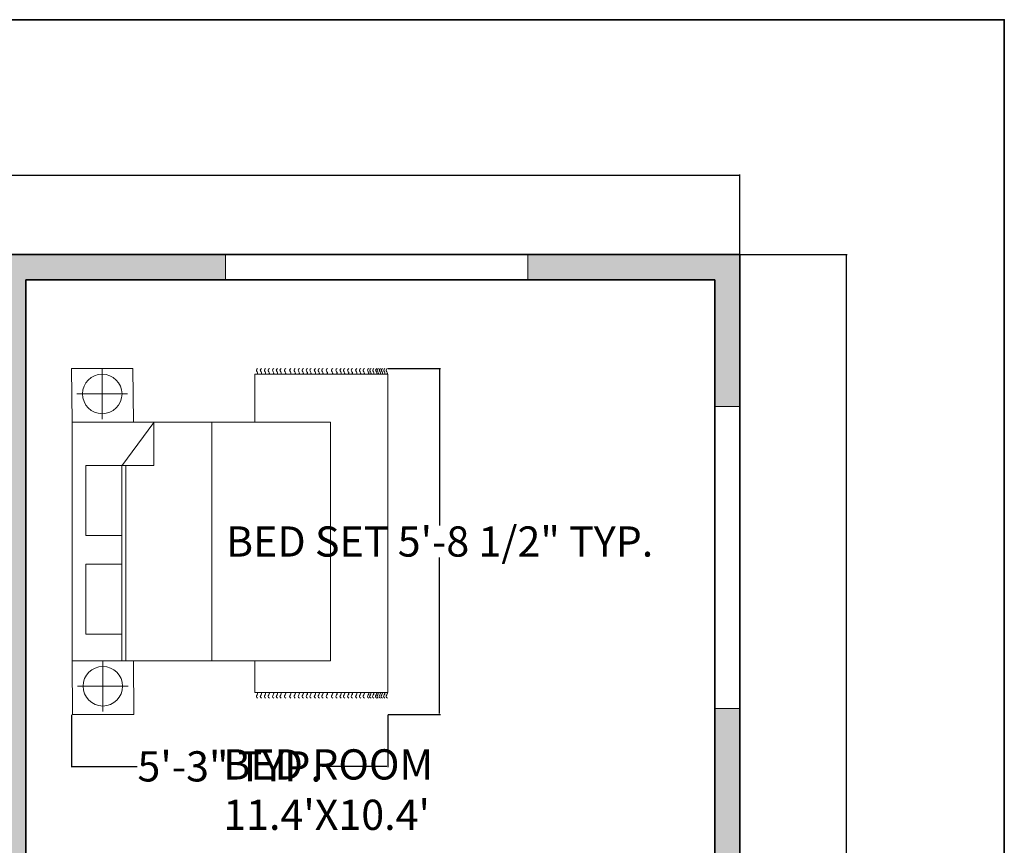
# Model space of a CAD drawing. Units: inches. Extents: x 717 to 1167, y 2046 to 2594.
# Tile 6 of 6: x 972 to 1167, y 2430 to 2594. Entities that reach past the tile are written whole.
import ezdxf

# ---------------------------------------------------------------- set-up
doc = ezdxf.new("R2010")
doc.units = ezdxf.units.IN
doc.header["$MEASUREMENT"] = 0
for name, color, linetype, lineweight in [('A-ANNO-DIMS', 2, 'Continuous', 18), ('A-ANNO-TTLB', 7, 'Continuous', 35), ('A-AREA-IDEN', 7, 'Continuous', 18), ('A-FURN', 8, 'Continuous', 18), ('A-GLAZ', 4, 'Continuous', 18), ('A-WALL', 7, 'Continuous', 35), ('A-WALL-PATT', 140, 'Continuous', 13)]:
    doc.layers.add(name, color=color, linetype=linetype, lineweight=lineweight)
doc.styles.get("Standard").update_dxf_attribs({"font": 'arial.ttf'})
doc.dimstyles.get("Standard").update_dxf_attribs({"dimtxt": 6, "dimasz": 0.18, "dimexe": 0.18, "dimexo": 0.0625, "dimgap": 0.09, "dimtad": 0, "dimtih": 1, "dimtoh": 1, "dimdec": 1, "dimzin": 0, "dimdsep": 46, "dimlunit": 3, "dimtxsty": 'Standard', "dimcen": 0.09, "dimadec": 0, "dimazin": 0, "dimtfac": 1, "dimtdec": 1, "dimtofl": 0, "dimtmove": 0, "dimatfit": 3, "dimfxl": 1, "dimtolj": 1, "dimtzin": 0, "dimarcsym": 0})

# ---------------------------------------------------------------- blocks, each defined once
blk = doc.blocks.new('*D4')
at = {"layer": 'A-ANNO-DIMS', "color": 0, "lineweight": -2, "transparency": 16777216}
for p, q in [((754.71, 2547.63), (754.71, 2563.46)), ((754.89, 2563.28), (929.54, 2563.28)), ((1114.53, 2563.28), (939.89, 2563.28)), ((1114.71, 2547.63), (1114.71, 2563.46))]:
    blk.add_line(p, q, dxfattribs=at)
at = {"layer": 'A-ANNO-DIMS', "color": 0, "transparency": 16777216}
for points in [[(754.89, 2563.31), (754.89, 2563.25), (754.71, 2563.28)], [(1114.53, 2563.31), (1114.53, 2563.25), (1114.71, 2563.28)]]:
    blk.add_solid(points, dxfattribs=at)
at = {"layer": 'Defpoints', "color": 0, "transparency": 16777216}
for p in [(1114.71, 2563.28), (754.71, 2547.57), (1114.71, 2547.57)]:
    blk.add_point(p, dxfattribs=at)
at = {"layer": 'A-ANNO-DIMS', "color": 0, "transparency": 16777216, "insert": (934.71, 2563.28), "char_height": 6, "attachment_point": 5}
blk.add_mtext("\\A1;30'", dxfattribs=at)
blk = doc.blocks.new('*D5')
at = {"layer": 'A-ANNO-DIMS', "color": 0, "lineweight": -2, "transparency": 16777216}
for p, q in [((1114.78, 2547.57), (1135.98, 2547.57)), ((1135.8, 2547.39), (1135.8, 2316.73)), ((1135.8, 2079.75), (1135.8, 2310.41)), ((1114.78, 2079.57), (1135.98, 2079.57))]:
    blk.add_line(p, q, dxfattribs=at)
at = {"layer": 'A-ANNO-DIMS', "color": 0, "transparency": 16777216}
for points in [[(1135.77, 2547.39), (1135.83, 2547.39), (1135.8, 2547.57)], [(1135.77, 2079.75), (1135.83, 2079.75), (1135.8, 2079.57)]]:
    blk.add_solid(points, dxfattribs=at)
at = {"layer": 'Defpoints', "color": 0, "transparency": 16777216}
for p in [(1114.71, 2547.57), (1114.71, 2079.57), (1135.8, 2079.57)]:
    blk.add_point(p, dxfattribs=at)
at = {"layer": 'A-ANNO-DIMS', "color": 0, "transparency": 16777216, "insert": (1135.8, 2313.57), "char_height": 6, "attachment_point": 5}
blk.add_mtext("\\A1;39'", dxfattribs=at)
blk = doc.blocks.new('BED-DOUBLE-WITH-NIGHTSTANDS')
for p, q in [((6.09, 68.68), (6.09, 58.62)), ((36.42, 67.59), (62.78, 67.59)), ((36.42, 58.05), (36.42, 67.59)), ((62.78, 67.59), (62.78, 4.35)), ((1.07, 63.65), (11.12, 63.65)), ((9.97, 49.39), (16.32, 58)), ((16.32, 49.44), (16.32, 58)), ((27.82, 58.05), (27.82, 10.63)), ((9.97, 49.44), (16.32, 49.44)), ((9.97, 49.39), (9.97, 10.63)), ((10.78, 49.44), (10.78, 10.63)), ((6.2, 10.63), (6.2, 0.57)), ((36.42, 4.35), (36.42, 10.65)), ((1.17, 5.6), (11.22, 5.6)), ((62.78, 4.35), (36.42, 4.35))]:
    blk.add_line(p, q)
for points in [[(12.29, 58.05), (12.19, 68.68), (0, 68.68), (0.1, 58.05)], [(0.1, 58.05), (51.42, 58.05), (51.42, 10.63), (0.1, 10.63)], [(2.8, 49.44), (9.97, 49.44), (9.97, 35.55), (2.8, 35.55)], [(2.8, 29.88), (9.97, 29.88), (9.97, 15.98), (2.8, 15.98)], [(12.39, 0), (12.29, 10.63), (0.1, 10.63), (0.21, 0)]]:
    blk.add_lwpolyline(points, close=True)
for centre in [(6.09, 63.65), (6.2, 5.6)]:
    blk.add_circle(centre, 3.92)
for points, knots in [([(36.95, 68.71), (36.83, 68.61), (36.59, 68.42), (36.83, 68.08), (37, 67.8), (36.89, 67.65), (36.85, 67.58)], [0, 0, 0, 0, 0.400747, 0.791423, 1.067667, 1.29709, 1.29709, 1.29709, 1.29709]), ([(37.73, 68.71), (37.61, 68.61), (37.37, 68.42), (37.61, 68.08), (37.78, 67.8), (37.67, 67.65), (37.62, 67.58)], [0, 0, 0, 0, 0.400747, 0.791423, 1.067667, 1.29709, 1.29709, 1.29709, 1.29709]), ([(38.54, 68.71), (38.42, 68.61), (38.18, 68.42), (38.42, 68.08), (38.59, 67.8), (38.49, 67.65), (38.44, 67.58)], [0, 0, 0, 0, 0.400747, 0.791423, 1.067667, 1.29709, 1.29709, 1.29709, 1.29709]), ([(39.27, 68.71), (39.15, 68.61), (38.91, 68.42), (39.15, 68.08), (39.32, 67.8), (39.22, 67.65), (39.17, 67.58)], [0, 0, 0, 0, 0.400747, 0.791423, 1.067667, 1.29709, 1.29709, 1.29709, 1.29709]), ([(40.15, 68.71), (40.03, 68.61), (39.79, 68.42), (40.03, 68.08), (40.2, 67.8), (40.1, 67.65), (40.05, 67.58)], [0, 0, 0, 0, 0.400747, 0.791423, 1.067667, 1.29709, 1.29709, 1.29709, 1.29709]), ([(40.91, 68.71), (40.78, 68.61), (40.54, 68.42), (40.78, 68.08), (40.96, 67.8), (40.85, 67.65), (40.8, 67.58)], [0, 0, 0, 0, 0.400747, 0.791423, 1.067667, 1.29709, 1.29709, 1.29709, 1.29709]), ([(41.63, 68.71), (41.51, 68.61), (41.27, 68.42), (41.51, 68.08), (41.69, 67.8), (41.58, 67.65), (41.53, 67.58)], [0, 0, 0, 0, 0.400747, 0.791423, 1.067667, 1.29709, 1.29709, 1.29709, 1.29709]), ([(42.52, 68.71), (42.39, 68.61), (42.16, 68.42), (42.39, 68.08), (42.57, 67.8), (42.46, 67.65), (42.41, 67.58)], [0, 0, 0, 0, 0.400747, 0.791423, 1.067667, 1.29709, 1.29709, 1.29709, 1.29709]), ([(43.55, 68.71), (43.43, 68.61), (43.19, 68.42), (43.43, 68.08), (43.6, 67.8), (43.5, 67.65), (43.45, 67.58)], [0, 0, 0, 0, 0.400747, 0.791423, 1.067667, 1.29709, 1.29709, 1.29709, 1.29709]), ([(44.43, 68.71), (44.31, 68.61), (44.07, 68.42), (44.31, 68.08), (44.49, 67.8), (44.38, 67.65), (44.33, 67.58)], [0, 0, 0, 0, 0.400747, 0.791423, 1.067667, 1.29709, 1.29709, 1.29709, 1.29709]), ([(45.25, 68.71), (45.13, 68.61), (44.89, 68.42), (45.13, 68.08), (45.3, 67.8), (45.2, 67.65), (45.15, 67.58)], [0, 0, 0, 0, 0.400747, 0.791423, 1.067667, 1.29709, 1.29709, 1.29709, 1.29709]), ([(46.03, 68.71), (45.91, 68.61), (45.67, 68.42), (45.91, 68.08), (46.08, 67.8), (45.97, 67.65), (45.92, 67.58)], [0, 0, 0, 0, 0.400747, 0.791423, 1.067667, 1.29709, 1.29709, 1.29709, 1.29709]), ([(46.84, 68.71), (46.72, 68.61), (46.48, 68.42), (46.72, 68.08), (46.9, 67.8), (46.79, 67.65), (46.74, 67.58)], [0, 0, 0, 0, 0.400747, 0.791423, 1.067667, 1.29709, 1.29709, 1.29709, 1.29709]), ([(47.57, 68.71), (47.45, 68.61), (47.21, 68.42), (47.45, 68.08), (47.62, 67.8), (47.52, 67.65), (47.47, 67.58)], [0, 0, 0, 0, 0.400747, 0.791423, 1.067667, 1.29709, 1.29709, 1.29709, 1.29709]), ([(48.45, 68.71), (48.33, 68.61), (48.09, 68.42), (48.33, 68.08), (48.51, 67.8), (48.4, 67.65), (48.35, 67.58)], [0, 0, 0, 0, 0.400747, 0.791423, 1.067667, 1.29709, 1.29709, 1.29709, 1.29709]), ([(49.21, 68.71), (49.08, 68.61), (48.85, 68.42), (49.08, 68.08), (49.26, 67.8), (49.15, 67.65), (49.1, 67.58)], [0, 0, 0, 0, 0.400747, 0.791423, 1.067667, 1.29709, 1.29709, 1.29709, 1.29709]), ([(49.93, 68.71), (49.81, 68.61), (49.57, 68.42), (49.81, 68.08), (49.99, 67.8), (49.88, 67.65), (49.83, 67.58)], [0, 0, 0, 0, 0.400747, 0.791423, 1.067667, 1.29709, 1.29709, 1.29709, 1.29709]), ([(50.82, 68.71), (50.69, 68.61), (50.46, 68.42), (50.69, 68.08), (50.87, 67.8), (50.76, 67.65), (50.71, 67.58)], [0, 0, 0, 0, 0.400747, 0.791423, 1.067667, 1.29709, 1.29709, 1.29709, 1.29709]), ([(51.85, 68.71), (51.73, 68.61), (51.49, 68.42), (51.73, 68.08), (51.9, 67.8), (51.8, 67.65), (51.75, 67.58)], [0, 0, 0, 0, 0.400747, 0.791423, 1.067667, 1.29709, 1.29709, 1.29709, 1.29709]), ([(52.74, 68.71), (52.61, 68.61), (52.37, 68.42), (52.61, 68.08), (52.79, 67.8), (52.68, 67.65), (52.63, 67.58)], [0, 0, 0, 0, 0.400747, 0.791423, 1.067667, 1.29709, 1.29709, 1.29709, 1.29709]), ([(53.55, 68.71), (53.43, 68.61), (53.19, 68.42), (53.43, 68.08), (53.6, 67.8), (53.5, 67.65), (53.45, 67.58)], [0, 0, 0, 0, 0.400747, 0.791423, 1.067667, 1.29709, 1.29709, 1.29709, 1.29709]), ([(54.24, 68.71), (54.12, 68.61), (53.88, 68.42), (54.12, 68.08), (54.29, 67.8), (54.19, 67.65), (54.14, 67.58)], [0, 0, 0, 0, 0.400747, 0.791423, 1.067667, 1.29709, 1.29709, 1.29709, 1.29709]), ([(55.06, 68.71), (54.94, 68.61), (54.7, 68.42), (54.94, 68.08), (55.11, 67.8), (55, 67.65), (54.95, 67.58)], [0, 0, 0, 0, 0.400747, 0.791423, 1.067667, 1.29709, 1.29709, 1.29709, 1.29709]), ([(55.78, 68.71), (55.66, 68.61), (55.42, 68.42), (55.66, 68.08), (55.84, 67.8), (55.73, 67.65), (55.68, 67.58)], [0, 0, 0, 0, 0.400747, 0.791423, 1.067667, 1.29709, 1.29709, 1.29709, 1.29709]), ([(56.67, 68.71), (56.55, 68.61), (56.31, 68.42), (56.55, 68.08), (56.72, 67.8), (56.61, 67.65), (56.56, 67.58)], [0, 0, 0, 0, 0.400747, 0.791423, 1.067667, 1.29709, 1.29709, 1.29709, 1.29709]), ([(57.42, 68.71), (57.3, 68.61), (57.06, 68.42), (57.3, 68.08), (57.47, 67.8), (57.36, 67.65), (57.32, 67.58)], [0, 0, 0, 0, 0.400747, 0.791423, 1.067667, 1.29709, 1.29709, 1.29709, 1.29709]), ([(58.15, 68.71), (58.03, 68.61), (57.79, 68.42), (58.03, 68.08), (58.2, 67.8), (58.1, 67.66), (58.05, 67.59)], [0, 0, 0, 0, 0.400747, 0.791423, 1.067667, 1.283686, 1.283686, 1.283686, 1.283686]), ([(59.03, 68.71), (58.91, 68.61), (58.67, 68.42), (58.91, 68.08), (59.08, 67.8), (58.98, 67.66), (58.93, 67.59)], [0, 0, 0, 0, 0.400747, 0.791423, 1.067667, 1.283686, 1.283686, 1.283686, 1.283686]), ([(59.46, 68.71), (59.34, 68.61), (59.09, 68.42), (59.34, 68.08), (59.51, 67.8), (59.41, 67.66), (59.36, 67.59)], [0, 0, 0, 0, 0.402903, 0.794912, 1.071156, 1.287177, 1.287177, 1.287177, 1.287177]), ([(60.05, 68.71), (59.93, 68.61), (59.69, 68.42), (59.93, 68.08), (60.1, 67.8), (60, 67.66), (59.96, 67.59)], [0, 0, 0, 0, 0.400747, 0.791423, 1.067667, 1.283686, 1.283686, 1.283686, 1.283686]), ([(60.63, 68.71), (60.51, 68.61), (60.27, 68.42), (60.51, 68.08), (60.68, 67.8), (60.58, 67.66), (60.53, 67.59)], [0, 0, 0, 0, 0.400747, 0.791423, 1.067667, 1.283686, 1.283686, 1.283686, 1.283686]), ([(60.94, 68.71), (60.82, 68.61), (60.58, 68.42), (60.81, 68.08), (60.99, 67.8), (60.89, 67.66), (60.84, 67.59)], [0, 0, 0, 0, 0.400747, 0.791423, 1.067667, 1.283686, 1.283686, 1.283686, 1.283686]), ([(61.36, 68.71), (61.23, 68.61), (60.99, 68.42), (61.23, 68.08), (61.41, 67.8), (61.3, 67.65), (61.25, 67.58)], [0, 0, 0, 0, 0.400747, 0.791423, 1.067667, 1.29709, 1.29709, 1.29709, 1.29709]), ([(61.75, 68.71), (61.63, 68.61), (61.39, 68.42), (61.63, 68.08), (61.8, 67.8), (61.7, 67.65), (61.65, 67.58)], [0, 0, 0, 0, 0.400747, 0.791423, 1.067667, 1.29709, 1.29709, 1.29709, 1.29709]), ([(62.24, 68.71), (62.12, 68.61), (61.88, 68.42), (62.12, 68.08), (62.29, 67.8), (62.18, 67.65), (62.13, 67.58)], [0, 0, 0, 0, 0.400747, 0.791423, 1.067667, 1.29709, 1.29709, 1.29709, 1.29709]), ([(62.71, 68.71), (62.59, 68.61), (62.35, 68.42), (62.59, 68.08), (62.76, 67.8), (62.66, 67.65), (62.61, 67.58)], [0, 0, 0, 0, 0.400747, 0.791423, 1.067667, 1.29709, 1.29709, 1.29709, 1.29709]), ([(36.95, 3.23), (36.83, 3.32), (36.59, 3.52), (36.83, 3.86), (37, 4.14), (36.89, 4.29), (36.85, 4.35)], [0, 0, 0, 0, 0.400747, 0.791423, 1.067667, 1.29709, 1.29709, 1.29709, 1.29709]), ([(37.73, 3.23), (37.61, 3.32), (37.37, 3.52), (37.61, 3.86), (37.78, 4.14), (37.67, 4.29), (37.62, 4.35)], [0, 0, 0, 0, 0.400747, 0.791423, 1.067667, 1.29709, 1.29709, 1.29709, 1.29709]), ([(38.54, 3.23), (38.42, 3.32), (38.18, 3.52), (38.42, 3.86), (38.59, 4.14), (38.49, 4.29), (38.44, 4.35)], [0, 0, 0, 0, 0.400747, 0.791423, 1.067667, 1.29709, 1.29709, 1.29709, 1.29709]), ([(39.27, 3.23), (39.15, 3.32), (38.91, 3.52), (39.15, 3.86), (39.32, 4.14), (39.22, 4.29), (39.17, 4.35)], [0, 0, 0, 0, 0.400747, 0.791423, 1.067667, 1.29709, 1.29709, 1.29709, 1.29709]), ([(40.15, 3.23), (40.03, 3.32), (39.79, 3.52), (40.03, 3.86), (40.2, 4.14), (40.1, 4.29), (40.05, 4.35)], [0, 0, 0, 0, 0.400747, 0.791423, 1.067667, 1.29709, 1.29709, 1.29709, 1.29709]), ([(40.91, 3.23), (40.78, 3.32), (40.54, 3.52), (40.78, 3.86), (40.96, 4.14), (40.85, 4.29), (40.8, 4.35)], [0, 0, 0, 0, 0.400747, 0.791423, 1.067667, 1.29709, 1.29709, 1.29709, 1.29709]), ([(41.63, 3.23), (41.51, 3.32), (41.27, 3.52), (41.51, 3.86), (41.69, 4.14), (41.58, 4.29), (41.53, 4.35)], [0, 0, 0, 0, 0.400747, 0.791423, 1.067667, 1.29709, 1.29709, 1.29709, 1.29709]), ([(42.52, 3.23), (42.39, 3.32), (42.16, 3.52), (42.39, 3.86), (42.57, 4.14), (42.46, 4.29), (42.41, 4.35)], [0, 0, 0, 0, 0.400747, 0.791423, 1.067667, 1.29709, 1.29709, 1.29709, 1.29709]), ([(43.55, 3.23), (43.43, 3.32), (43.19, 3.52), (43.43, 3.86), (43.6, 4.14), (43.5, 4.29), (43.45, 4.35)], [0, 0, 0, 0, 0.400747, 0.791423, 1.067667, 1.29709, 1.29709, 1.29709, 1.29709]), ([(44.43, 3.23), (44.31, 3.32), (44.07, 3.52), (44.31, 3.86), (44.49, 4.14), (44.38, 4.29), (44.33, 4.35)], [0, 0, 0, 0, 0.400747, 0.791423, 1.067667, 1.29709, 1.29709, 1.29709, 1.29709]), ([(45.25, 3.23), (45.13, 3.32), (44.89, 3.52), (45.13, 3.86), (45.3, 4.14), (45.2, 4.29), (45.15, 4.35)], [0, 0, 0, 0, 0.400747, 0.791423, 1.067667, 1.29709, 1.29709, 1.29709, 1.29709]), ([(46.03, 3.23), (45.91, 3.32), (45.67, 3.52), (45.91, 3.86), (46.08, 4.14), (45.97, 4.29), (45.92, 4.35)], [0, 0, 0, 0, 0.400747, 0.791423, 1.067667, 1.29709, 1.29709, 1.29709, 1.29709]), ([(46.84, 3.23), (46.72, 3.32), (46.48, 3.52), (46.72, 3.86), (46.9, 4.14), (46.79, 4.29), (46.74, 4.35)], [0, 0, 0, 0, 0.400747, 0.791423, 1.067667, 1.29709, 1.29709, 1.29709, 1.29709]), ([(47.57, 3.23), (47.45, 3.32), (47.21, 3.52), (47.45, 3.86), (47.62, 4.14), (47.52, 4.29), (47.47, 4.35)], [0, 0, 0, 0, 0.400747, 0.791423, 1.067667, 1.29709, 1.29709, 1.29709, 1.29709]), ([(48.45, 3.23), (48.33, 3.32), (48.09, 3.52), (48.33, 3.86), (48.51, 4.14), (48.4, 4.29), (48.35, 4.35)], [0, 0, 0, 0, 0.400747, 0.791423, 1.067667, 1.29709, 1.29709, 1.29709, 1.29709]), ([(49.21, 3.23), (49.08, 3.32), (48.85, 3.52), (49.08, 3.86), (49.26, 4.14), (49.15, 4.29), (49.1, 4.35)], [0, 0, 0, 0, 0.400747, 0.791423, 1.067667, 1.29709, 1.29709, 1.29709, 1.29709]), ([(49.93, 3.23), (49.81, 3.32), (49.57, 3.52), (49.81, 3.86), (49.99, 4.14), (49.88, 4.29), (49.83, 4.35)], [0, 0, 0, 0, 0.400747, 0.791423, 1.067667, 1.29709, 1.29709, 1.29709, 1.29709]), ([(50.82, 3.23), (50.69, 3.32), (50.46, 3.52), (50.69, 3.86), (50.87, 4.14), (50.76, 4.29), (50.71, 4.35)], [0, 0, 0, 0, 0.400747, 0.791423, 1.067667, 1.29709, 1.29709, 1.29709, 1.29709]), ([(51.85, 3.23), (51.73, 3.32), (51.49, 3.52), (51.73, 3.86), (51.9, 4.14), (51.8, 4.29), (51.75, 4.35)], [0, 0, 0, 0, 0.400747, 0.791423, 1.067667, 1.29709, 1.29709, 1.29709, 1.29709]), ([(52.74, 3.23), (52.61, 3.32), (52.37, 3.52), (52.61, 3.86), (52.79, 4.14), (52.68, 4.29), (52.63, 4.35)], [0, 0, 0, 0, 0.400747, 0.791423, 1.067667, 1.29709, 1.29709, 1.29709, 1.29709]), ([(53.55, 3.23), (53.43, 3.32), (53.19, 3.52), (53.43, 3.86), (53.6, 4.14), (53.5, 4.29), (53.45, 4.35)], [0, 0, 0, 0, 0.400747, 0.791423, 1.067667, 1.29709, 1.29709, 1.29709, 1.29709]), ([(54.24, 3.23), (54.12, 3.32), (53.88, 3.52), (54.12, 3.86), (54.29, 4.14), (54.19, 4.29), (54.14, 4.35)], [0, 0, 0, 0, 0.400747, 0.791423, 1.067667, 1.29709, 1.29709, 1.29709, 1.29709]), ([(55.06, 3.23), (54.94, 3.32), (54.7, 3.52), (54.94, 3.86), (55.11, 4.14), (55, 4.29), (54.95, 4.35)], [0, 0, 0, 0, 0.400747, 0.791423, 1.067667, 1.29709, 1.29709, 1.29709, 1.29709]), ([(55.78, 3.23), (55.66, 3.32), (55.42, 3.52), (55.66, 3.86), (55.84, 4.14), (55.73, 4.29), (55.68, 4.35)], [0, 0, 0, 0, 0.400747, 0.791423, 1.067667, 1.29709, 1.29709, 1.29709, 1.29709]), ([(56.67, 3.23), (56.55, 3.32), (56.31, 3.52), (56.55, 3.86), (56.72, 4.14), (56.61, 4.29), (56.56, 4.35)], [0, 0, 0, 0, 0.400747, 0.791423, 1.067667, 1.29709, 1.29709, 1.29709, 1.29709]), ([(57.42, 3.23), (57.3, 3.32), (57.06, 3.52), (57.3, 3.86), (57.47, 4.14), (57.36, 4.29), (57.32, 4.35)], [0, 0, 0, 0, 0.400747, 0.791423, 1.067667, 1.29709, 1.29709, 1.29709, 1.29709]), ([(58.15, 3.23), (58.03, 3.32), (57.79, 3.52), (58.03, 3.86), (58.2, 4.14), (58.09, 4.29), (58.04, 4.35)], [0, 0, 0, 0, 0.400747, 0.791423, 1.067667, 1.29709, 1.29709, 1.29709, 1.29709]), ([(59.03, 3.23), (58.91, 3.32), (58.67, 3.52), (58.91, 3.86), (59.08, 4.14), (58.98, 4.29), (58.93, 4.35)], [0, 0, 0, 0, 0.400747, 0.791423, 1.067667, 1.29709, 1.29709, 1.29709, 1.29709]), ([(59.46, 3.23), (59.33, 3.32), (59.08, 3.51), (59.34, 3.86), (59.51, 4.14), (59.4, 4.29), (59.36, 4.35)], [0, 0, 0, 0, 0.407265, 0.802015, 1.07826, 1.307683, 1.307683, 1.307683, 1.307683]), ([(60.03, 3.23), (59.9, 3.32), (59.67, 3.52), (59.9, 3.86), (60.08, 4.14), (59.97, 4.29), (59.92, 4.35)], [0, 0, 0, 0, 0.400747, 0.791423, 1.067667, 1.29709, 1.29709, 1.29709, 1.29709]), ([(60.6, 3.23), (60.48, 3.32), (60.24, 3.52), (60.48, 3.86), (60.65, 4.14), (60.54, 4.29), (60.5, 4.35)], [0, 0, 0, 0, 0.400747, 0.791423, 1.067667, 1.29709, 1.29709, 1.29709, 1.29709]), ([(60.91, 3.23), (60.79, 3.32), (60.55, 3.52), (60.79, 3.86), (60.96, 4.14), (60.85, 4.29), (60.81, 4.35)], [0, 0, 0, 0, 0.400747, 0.791423, 1.067667, 1.29709, 1.29709, 1.29709, 1.29709]), ([(61.33, 3.23), (61.21, 3.32), (60.97, 3.52), (61.21, 3.86), (61.38, 4.14), (61.27, 4.29), (61.22, 4.35)], [0, 0, 0, 0, 0.400747, 0.791423, 1.067667, 1.29709, 1.29709, 1.29709, 1.29709]), ([(61.72, 3.23), (61.6, 3.32), (61.36, 3.52), (61.6, 3.86), (61.78, 4.14), (61.67, 4.29), (61.62, 4.35)], [0, 0, 0, 0, 0.400747, 0.791423, 1.067667, 1.29709, 1.29709, 1.29709, 1.29709]), ([(62.21, 3.23), (62.09, 3.32), (61.85, 3.52), (62.09, 3.86), (62.26, 4.14), (62.15, 4.29), (62.11, 4.35)], [0, 0, 0, 0, 0.400747, 0.791423, 1.067667, 1.29709, 1.29709, 1.29709, 1.29709]), ([(62.71, 3.23), (62.59, 3.32), (62.35, 3.52), (62.59, 3.86), (62.76, 4.14), (62.66, 4.29), (62.61, 4.35)], [0, 0, 0, 0, 0.400747, 0.791423, 1.067667, 1.29709, 1.29709, 1.29709, 1.29709])]:
    blk.add_open_spline(points, degree=3, knots=knots)
blk = doc.blocks.new('WINDOW-60IN')
for p, q in [((0, 5), (0, 0)), ((60, 5), (0, 5)), ((60, 0), (60, 5)), ((0, 0), (60, 0))]:
    blk.add_line(p, q)
blk = doc.blocks.new('*D17')
at = {"layer": 'A-ANNO-DIMS', "color": 0, "lineweight": -2, "transparency": 16777216}
for p, q in [((1044.83, 2524.95), (1055.25, 2524.95)), ((1055.07, 2524.77), (1055.07, 2493.78)), ((1055.07, 2456.42), (1055.07, 2487.4)), ((1044.83, 2456.24), (1055.25, 2456.24))]:
    blk.add_line(p, q, dxfattribs=at)
at = {"layer": 'A-ANNO-DIMS', "color": 0, "transparency": 16777216}
for points in [[(1055.04, 2524.77), (1055.1, 2524.77), (1055.07, 2524.95)], [(1055.04, 2456.42), (1055.1, 2456.42), (1055.07, 2456.24)]]:
    blk.add_solid(points, dxfattribs=at)
at = {"layer": 'Defpoints', "color": 0, "transparency": 16777216}
for p in [(1044.76, 2524.95), (1055.07, 2524.95), (1044.76, 2456.24)]:
    blk.add_point(p, dxfattribs=at)
at = {"layer": 'A-ANNO-DIMS', "color": 0, "transparency": 16777216, "insert": (1055.07, 2490.59), "char_height": 6, "attachment_point": 5}
blk.add_mtext('\\A1;BED SET 5\'-8 1/2" TYP.', dxfattribs=at)
blk = doc.blocks.new('*D18')
at = {"layer": 'A-ANNO-DIMS', "color": 0, "lineweight": -2, "transparency": 16777216}
for p, q in [((981.98, 2456.18), (981.98, 2445.75)), ((1044.76, 2456.18), (1044.76, 2445.75)), ((982.16, 2445.93), (995, 2445.93)), ((1044.58, 2445.93), (1031.75, 2445.93))]:
    blk.add_line(p, q, dxfattribs=at)
at = {"layer": 'A-ANNO-DIMS', "color": 0, "transparency": 16777216}
for points in [[(982.16, 2445.96), (982.16, 2445.9), (981.98, 2445.93)], [(1044.58, 2445.96), (1044.58, 2445.9), (1044.76, 2445.93)]]:
    blk.add_solid(points, dxfattribs=at)
at = {"layer": 'Defpoints', "color": 0, "transparency": 16777216}
for p in [(981.98, 2456.24), (1044.76, 2456.24), (1044.76, 2445.93)]:
    blk.add_point(p, dxfattribs=at)
at = {"layer": 'A-ANNO-DIMS', "color": 0, "transparency": 16777216, "insert": (1013.37, 2445.93), "char_height": 6, "attachment_point": 5}
blk.add_mtext('\\A1;5\'-3" TYP.', dxfattribs=at)

msp = doc.modelspace()

# ---------------------------------------------------------------- hatches: boundary and pattern name
at = {"layer": 'A-WALL-PATT'}
h = msp.add_hatch(color=256, dxfattribs=at)
h.dxf.hatch_style = 1
h.paths.add_polyline_path([(796.2, 2547.57), (754.71, 2547.57), (754.71, 2325.38), (759.71, 2325.38), (759.71, 2357.37), (840.31, 2357.37), (840.31, 2362.37), (759.71, 2362.37), (759.71, 2412.77), (835.31, 2412.77), (835.31, 2386.37), (840.31, 2386.37), (840.31, 2412.77), (901.51, 2412.77), (901.51, 2417.77), (759.71, 2417.77), (759.71, 2542.57), (796.2, 2542.57)])
h.paths.add_polyline_path([(913.34, 2547.57), (856.2, 2547.57), (856.2, 2542.57), (896.51, 2542.57), (896.51, 2453.77), (901.51, 2453.77), (901.51, 2542.57), (913.34, 2542.57)])
h.paths.add_polyline_path([(1012.57, 2547.57), (949.34, 2547.57), (949.34, 2542.57), (967.91, 2542.57), (967.91, 2412.77), (972.91, 2412.77), (972.91, 2542.57), (1012.57, 2542.57)])
h.paths.add_polyline_path([(1114.71, 2547.57), (1072.57, 2547.57), (1072.57, 2542.57), (1109.71, 2542.57), (1109.71, 2517.4), (1114.71, 2517.4)])
h.paths.add_polyline_path([(1114.71, 2457.4), (1109.71, 2457.4), (1109.71, 2393.68), (1114.71, 2393.68)])
h.paths.add_polyline_path([(1114.71, 2369.68), (1109.71, 2369.68), (1109.71, 2362.37), (1038.91, 2362.37), (1038.91, 2412.77), (1085.71, 2412.77), (1085.71, 2417.77), (1008.91, 2417.77), (1008.91, 2412.77), (1033.91, 2412.77), (1033.91, 2362.37), (916.31, 2362.37), (916.31, 2357.37), (1033.91, 2357.37), (1033.91, 2306.97), (1003.91, 2306.97), (1003.91, 2301.97), (1085.71, 2301.97), (1085.71, 2306.97), (1038.91, 2306.97), (1038.91, 2357.37), (1109.71, 2357.37), (1109.71, 2347.44), (1114.71, 2347.44)])
h.paths.add_polyline_path([(788.58, 2239.77), (759.71, 2239.77), (759.71, 2265.38), (754.71, 2265.38), (754.71, 2234.77), (788.58, 2234.77)])
h.paths.add_polyline_path([(880.31, 2362.37), (875.31, 2362.37), (875.31, 2239.77), (848.58, 2239.77), (848.58, 2234.77), (875.31, 2234.77), (875.31, 2079.57), (880.31, 2079.57)])
h.paths.add_polyline_path([(1008.91, 2265.97), (1003.91, 2265.97), (1003.91, 2127.77), (991.51, 2127.77), (991.51, 2122.77), (1003.91, 2122.77), (1003.91, 2079.57), (1036.96, 2079.57), (1036.96, 2084.57), (1008.91, 2084.57)])
h.paths.add_polyline_path([(931.51, 2127.77), (916.31, 2127.77), (916.31, 2122.77), (931.51, 2122.77)])
h.paths.add_polyline_path([(1114.71, 2162.57), (1109.71, 2162.57), (1109.71, 2084.57), (1096.96, 2084.57), (1096.96, 2079.57), (1114.71, 2079.57)])
h.paths.add_polyline_path([(1114.71, 2211.37), (1109.71, 2211.37), (1109.71, 2191.57), (1044.91, 2191.57), (1044.91, 2186.57), (1114.71, 2186.57)])
h.paths.add_polyline_path([(1114.71, 2323.44), (1109.71, 2323.44), (1109.71, 2271.37), (1114.71, 2271.37)])

# ---------------------------------------------------------------- linework, layer by layer
at = {"layer": 'A-ANNO-TTLB'}
msp.add_lwpolyline([(719.86, 2594.22), (1167.21, 2594.22), (1167.21, 2050.08), (719.86, 2050.08)], close=True, dxfattribs=at)
at = {"layer": 'A-GLAZ'}
for p, q in [((1012.57, 2547.57), (1012.57, 2542.57)), ((1072.57, 2547.57), (1014.23, 2547.57)), ((1072.57, 2542.57), (1072.57, 2547.57)), ((1012.57, 2542.57), (1072.57, 2542.57))]:
    msp.add_line(p, q, dxfattribs=at)
at = {"layer": 'A-WALL'}
for p, q in [((754.71, 2547.57), (1114.71, 2547.57)), ((1114.71, 2547.57), (1114.71, 2079.57)), ((972.91, 2542.57), (972.91, 2412.77)), ((972.91, 2542.57), (1109.71, 2542.57)), ((1109.71, 2542.57), (1109.71, 2362.37))]:
    msp.add_line(p, q, dxfattribs=at)

# ---------------------------------------------------------------- block references
at = {"layer": 'A-FURN'}
msp.add_blockref('BED-DOUBLE-WITH-NIGHTSTANDS', (981.98, 2456.24), dxfattribs=at)
at = {"layer": 'A-GLAZ', "rotation": 270}
msp.add_blockref('WINDOW-60IN', (1109.71, 2517.4), dxfattribs=at)

# ---------------------------------------------------------------- texts
at = {"layer": 'A-AREA-IDEN', "insert": (1012.1, 2449.32), "char_height": 6, "attachment_point": 1}
msp.add_mtext_dynamic_manual_height_columns("BED ROOM\\P11.4'X10.4'", width=66.6171, gutter_width=30, heights=[0], dxfattribs=at)

# ---------------------------------------------------------------- dimensions: what is measured, and where the dimension line sits
at = {"layer": 'A-ANNO-DIMS'}
dim = msp.add_linear_dim(base=(1114.71, 2563.28), p1=(754.71, 2547.57), p2=(1114.71, 2547.57), dimstyle='Standard', override={"dimclrd": 0, "dimclre": 0, "dimclrt": 0}, dxfattribs=at)
dim.commit()
dim.dimension.update_dxf_attribs({"geometry": '*D4', "text_midpoint": (934.71, 2563.28)})
dim = msp.add_linear_dim(base=(1135.8, 2079.57), p1=(1114.71, 2547.57), p2=(1114.71, 2079.57), angle=90, dimstyle='Standard', override={"dimclrd": 0, "dimclre": 0, "dimclrt": 0}, dxfattribs=at)
dim.commit()
dim.dimension.update_dxf_attribs({"geometry": '*D5', "text_midpoint": (1135.8, 2313.57)})
dim = msp.add_linear_dim(base=(1055.07, 2524.95), p1=(1044.76, 2456.24), p2=(1044.76, 2524.95), angle=90, text='BED SET <> TYP.', dimstyle='Standard', override={"dimdec": 1, "dimlfac": 1, "dimrnd": 0, "dimzin": 1, "dimdsep": 46, "dimlunit": 4, "dimfrac": 2}, dxfattribs=at)
dim.commit()
dim.dimension.update_dxf_attribs({"geometry": '*D17', "text_midpoint": (1055.07, 2490.59)})
dim = msp.add_linear_dim(base=(1044.76, 2445.93), p1=(981.98, 2456.24), p2=(1044.76, 2456.24), text='<> TYP.', dimstyle='Standard', override={"dimdec": 1, "dimlfac": 1, "dimrnd": 0, "dimzin": 1, "dimdsep": 46, "dimlunit": 4, "dimfrac": 2}, dxfattribs=at)
dim.commit()
dim.dimension.update_dxf_attribs({"geometry": '*D18', "text_midpoint": (1013.37, 2445.93)})

doc.saveas('drawing.dxf')
